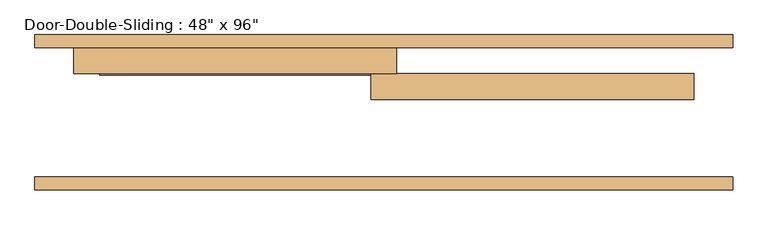
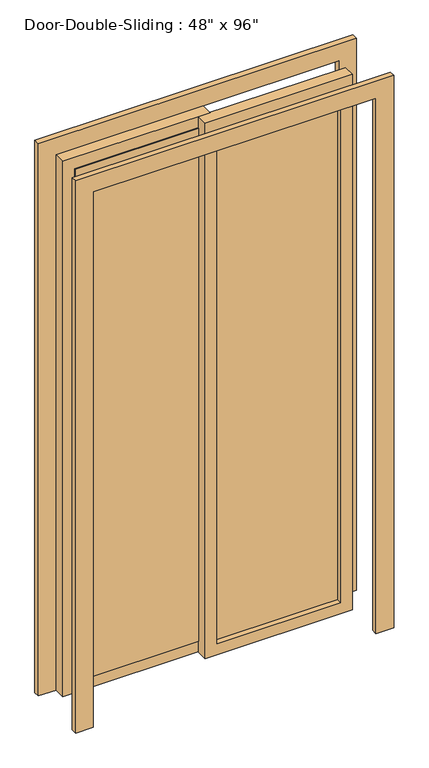
"""IFC4 building model written with IfcOpenShell, lengths in millimetres: door geometry."""

from ifc_helpers import new_model, si_unit, frame, origin, place, context, project, spatial, polyline, outline, extrude, source, transform, mapped, element, save


def door_ed536266(model_context):
    return source(origin(), model_context, "Body", "SweptSolid", [
        extrude(outline(polyline([(0.0, 685.8), (2514.6, 685.8), (2514.6, -685.8), (0.0, -685.8), (0.0, -609.6), (2438.4, -609.6), (2438.4, 609.6), (0.0, 609.6), (0.0, 685.8)])), frame((0.0, 254.0, 0.0), z_axis=(0.0, 1.0, 0.0), x_axis=(0.0, 0.0, 1.0)), (0.0, 0.0, 1.0), 25.4),
        extrude(outline(polyline([(0.0, -685.8), (0.0, -609.6), (2438.4, -609.6), (2438.4, 609.6), (0.0, 609.6), (0.0, 685.8), (2514.6, 685.8), (2514.6, -685.8), (0.0, -685.8)])), frame((0.0, -25.4, 0.0), z_axis=(0.0, 1.0, 0.0), x_axis=(0.0, 0.0, 1.0)), (0.0, 0.0, 1.0), 25.4),
        extrude(outline(polyline([(2438.4, 25.4), (2438.4, -609.6), (0.0, -609.6), (0.0, 25.4), (2438.4, 25.4)]), holes=[polyline([(2387.6, -25.4), (50.8, -25.4), (50.8, -558.8), (2387.6, -558.8), (2387.6, -25.4)])]), frame((0.0, 203.2, 0.0), z_axis=(0.0, 1.0, 0.0), x_axis=(0.0, 0.0, 1.0)), (0.0, 0.0, 1.0), 50.8),
        extrude(outline(polyline([(2438.4, -25.4), (0.0, -25.4), (0.0, 609.6), (2438.4, 609.6), (2438.4, -25.4)]), holes=[polyline([(2387.6, 25.4), (2387.6, 558.8), (50.8, 558.8), (50.8, 25.4), (2387.6, 25.4)])]), frame((0.0, 152.4, 0.0), z_axis=(0.0, 1.0, 0.0), x_axis=(0.0, 0.0, 1.0)), (0.0, 0.0, 1.0), 50.8),
        extrude(outline(polyline([(-25.4, 200.025), (-558.8, 200.025), (-558.8, 206.375), (-25.4, 206.375), (-25.4, 200.025)])), frame((0.0, 0.0, 50.8), z_axis=(0.0, 0.0, 1.0), x_axis=(1.0, 0.0, 0.0)), (0.0, 0.0, 1.0), 2336.8),
        extrude(outline(polyline([(25.4, 180.975), (558.8, 180.975), (558.8, 174.625), (25.4, 174.625), (25.4, 180.975)])), frame((0.0, 0.0, 50.8), z_axis=(0.0, 0.0, 1.0), x_axis=(1.0, 0.0, 0.0)), (0.0, 0.0, 1.0), 2336.8),
    ])


if __name__ == "__main__":
    model = new_model("IFC4")
    model_context = context("Model", 3, world=origin())
    ifc_project = project(units=[si_unit("LENGTHUNIT", "METRE", prefix="MILLI")], contexts=[model_context])
    site = spatial("IfcSite", under=ifc_project)
    building = spatial("IfcBuilding", under=site)
    placement = place(None, origin())
    door_shape = door_ed536266(model_context)
    element("IfcDoor", 1, ObjectType="Door-Double-Sliding : 48\" x 96\"", at=placement, inside=building, context=model_context, shape_type="MappedRepresentation", body=[
        mapped(door_shape, transform((0.0, 0.0, 0.0), x_axis=(1.0, 0.0, 0.0), y_axis=(0.0, 1.0, 0.0), z_axis=(0.0, 0.0, 1.0))),
    ])
    save(model, "model.ifc")

# Revit data of these elements
# Type "Door-Double-Sliding : 48\" x 96\""
#   Type Mark = "8"
#   Construction Type Id = "opn-d45"
#   Assembly Code = "C1020"
#   Analytic Construction = "Wood frame, double glass door "
#   Thickness = 0' - 2"
#   Thermal Resistance (R) = 1.8150 (h·ft²·°F)/BTU
#   Heat Transfer Coefficient (U) = 0.5510 BTU/(h·ft²·°F)
#   Height = 8' - 0"
#   Rail Width = 0' - 2"
#   Stiles = 0' - 2"
#   Trim Projection Ext = 0' - 1"
#   Trim Projection Int = 0' - 1"
#   Trim Width = 0' - 3"
#   Width = 4' - 0"
#   Define Thermal Properties by = 1
#   Glazing = Glass
#   Panel Material = Wood - Birch - Solid Stained Light Low Gloss
#   Trim Material = Paint - Sienna
#   Visual Light Transmittance = 0
#   Solar Heat Gain Coefficient = 0
#   Function = (empty or 0)
#   Wall Closure = (empty or 0)
# Element 1 (IfcDoor, "Door-Double-Sliding : 48\" x 96\"")
#   Materials on its faces: "Paint - Sienna", "Wood - Birch - Solid Stained Light Low Gloss", "Glass"
# Materials
#   "Glass": class "Glass", colour RGB 0 128 192, transparency 0.75, Description = "Soda Lime Glass", Cost = 0
#   "Wood - Birch - Solid Stained Light Low Gloss": class "Wood", colour RGB 210 159 95, transparency 0, Cost = 0
#   "Paint - Sienna": colour RGB 118 70 51, transparency 0, Cost = 0
